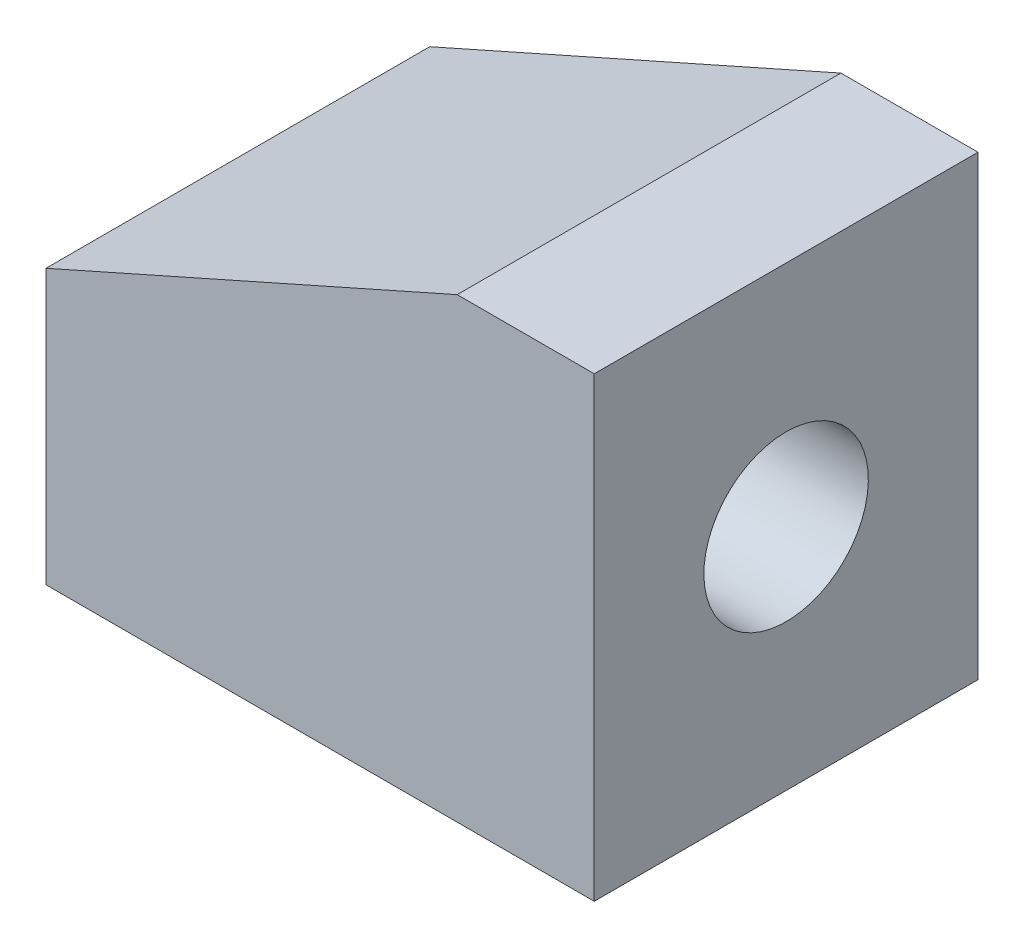
SolidWorks part; units mm, degrees
material "Plain Carbon Steel"
ref_plane "Front Plane" through (0, 0, 0) normal (0, 0, 1) x (1, 0, 0)
ref_plane "Top Plane" through (0, 0, 0) normal (0, 1, 0) x (1, 0, 0)
ref_plane "Right Plane" through (0, 0, 0) normal (1, 0, 0) x (0, 0, -1)
sketch "Block Profile Sketch" plane through (0, 0, 0) normal (0, 0, 1) x (1, 0, 0)
  line L0 (30, 0) -> (-30, 0)
  line L1 (-30, 0) -> (-30, 30)
  line L2 (-30, 30) -> (15, 50)
  line L3 (15, 50) -> (30, 50)
  line L4 (30, 50) -> (30, 0)
  point P4 (0, 0)
  dimension "D1" = 60
  dimension "D2" = 15
  dimension "D3" = 30
  dimension "D4" = 50
extrude "Block Body" add sketch "Block Profile Sketch" along normal mid plane 42
sketch "Bore Ø18 Sketch" plane through (30, 0, 0) normal (1, 0, 0) x (0, 0, -1)
  circle A0 centre (0, 25) radius 9
  dimension "D1" = 18
  dimension "D2" = 25
extrude "Bore Ø18 x 40 Deep" cut sketch "Bore Ø18 Sketch" against normal blind 40
cosmetic thread "Cosmetic Thread1" parameters "D2"=22
cosmetic thread "Cosmetic Thread2" parameters "D2"=20
